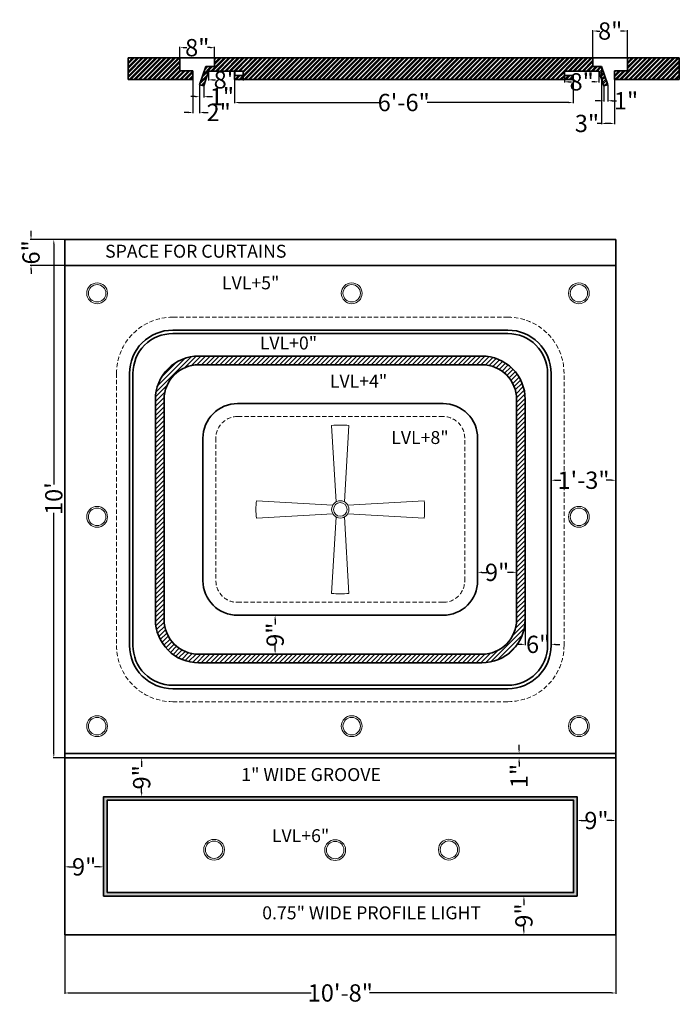
# Model space of a CAD drawing. Units: inches. Extents: x 412 to 565, y 109 to 337.
import ezdxf

# ---------------------------------------------------------------- set-up
doc = ezdxf.new("R2010")
doc.units = ezdxf.units.IN
doc.header["$LTSCALE"] = 2
doc.header["$MEASUREMENT"] = 0
doc.linetypes.add('DASHED', pattern=[0.75, 0.5, -0.25])
for name, color, linetype, lineweight in [('A-ANNO-DIMS', 2, 'Continuous', 18), ('A-ANNO-TEXT', 7, 'Continuous', 18), ('A-CLNG', 7, 'Continuous', 35), ('A-CLNG-LITE', 30, 'DASHED', 18), ('A-CLNG-PATT', 8, 'Continuous', 13), ('A-SECT', 7, 'Continuous', 35), ('E-FANS', 4, 'Continuous', 18), ('E-LITE', 3, 'Continuous', 18)]:
    doc.layers.add(name, color=color, linetype=linetype, lineweight=lineweight)
doc.styles.get("Standard").update_dxf_attribs({"font": 'arial.ttf'})
doc.dimstyles.get("Standard").update_dxf_attribs({"dimtxt": 4, "dimasz": 1, "dimexe": 0.18, "dimexo": 0.0625, "dimgap": 0.09, "dimtad": 0, "dimdec": 0, "dimzin": 0, "dimdsep": 46, "dimlunit": 4, "dimtxsty": 'Standard', "dimcen": 0.09, "dimadec": 0, "dimazin": 0, "dimtfac": 1, "dimtdec": 0, "dimtofl": 0, "dimtmove": 0, "dimatfit": 3, "dimfxl": 1, "dimtolj": 1, "dimtzin": 0, "dimarcsym": 0})

# ---------------------------------------------------------------- blocks, each defined once
blk = doc.blocks.new('*D1')
at = {"layer": 'A-ANNO-DIMS', "color": 0, "lineweight": -2, "transparency": 16777216}
for p, q in [((535.11, 254.83), (535.11, 229.97)), ((550.11, 236.95), (550.11, 229.97)), ((536.11, 230.15), (537.39, 230.15)), ((549.11, 230.15), (547.83, 230.15))]:
    blk.add_line(p, q, dxfattribs=at)
at = {"layer": 'A-ANNO-DIMS', "color": 0, "transparency": 16777216}
for points in [[(536.11, 230.31), (536.11, 229.98), (535.11, 230.15)], [(549.11, 230.31), (549.11, 229.98), (550.11, 230.15)]]:
    blk.add_solid(points, dxfattribs=at)
at = {"layer": 'Defpoints', "color": 0, "transparency": 16777216}
for p in [(535.11, 254.89), (550.11, 237.01), (535.11, 230.15)]:
    blk.add_point(p, dxfattribs=at)
at = {"layer": 'A-ANNO-DIMS', "color": 0, "transparency": 16777216, "insert": (542.61, 230.15), "char_height": 4, "attachment_point": 5}
blk.add_mtext('\\A1;1\'-3"', dxfattribs=at)
blk = doc.blocks.new('*D2')
at = {"layer": 'A-ANNO-DIMS', "color": 0, "lineweight": -2, "transparency": 16777216}
for p, q in [((529.11, 197.83), (529.11, 191.98)), ((528.11, 192.16), (527.11, 192.16)), ((535.11, 191.95), (535.11, 192.34)), ((536.11, 192.16), (537.11, 192.16))]:
    blk.add_line(p, q, dxfattribs=at)
at = {"layer": 'A-ANNO-DIMS', "color": 0, "transparency": 16777216}
for points in [[(528.11, 192.33), (528.11, 192), (529.11, 192.16)], [(536.11, 192.33), (536.11, 192), (535.11, 192.16)]]:
    blk.add_solid(points, dxfattribs=at)
at = {"layer": 'Defpoints', "color": 0, "transparency": 16777216}
for p in [(529.11, 197.89), (529.11, 192.16), (535.11, 191.89)]:
    blk.add_point(p, dxfattribs=at)
at = {"layer": 'A-ANNO-DIMS', "color": 0, "transparency": 16777216, "insert": (532.11, 192.16), "char_height": 4, "attachment_point": 5}
blk.add_mtext('\\A1;6"', dxfattribs=at)
blk = doc.blocks.new('*D3')
at = {"layer": 'A-ANNO-DIMS', "color": 0, "lineweight": -2, "transparency": 16777216}
for p, q in [((518.11, 206.95), (518.11, 209.01)), ((519.11, 208.83), (520.22, 208.83)), ((526.11, 208.83), (525, 208.83)), ((527.11, 197.95), (527.11, 209.01))]:
    blk.add_line(p, q, dxfattribs=at)
at = {"layer": 'A-ANNO-DIMS', "color": 0, "transparency": 16777216}
for points in [[(519.11, 209), (519.11, 208.67), (518.11, 208.83)], [(526.11, 209), (526.11, 208.67), (527.11, 208.83)]]:
    blk.add_solid(points, dxfattribs=at)
at = {"layer": 'Defpoints', "color": 0, "transparency": 16777216}
for p in [(527.11, 208.83), (518.11, 206.89), (527.11, 197.89)]:
    blk.add_point(p, dxfattribs=at)
at = {"layer": 'A-ANNO-DIMS', "color": 0, "transparency": 16777216, "insert": (522.61, 208.83), "char_height": 4, "attachment_point": 5}
blk.add_mtext('\\A1;9"', dxfattribs=at)
blk = doc.blocks.new('*D4')
at = {"layer": 'A-ANNO-DIMS', "color": 0, "lineweight": -2, "transparency": 16777216}
for p, q in [((462.57, 198.89), (471.4, 198.89)), ((471.22, 197.89), (471.22, 196.78)), ((471.22, 190.89), (471.22, 192)), ((453.57, 189.89), (471.4, 189.89))]:
    blk.add_line(p, q, dxfattribs=at)
at = {"layer": 'A-ANNO-DIMS', "color": 0, "transparency": 16777216}
for points in [[(471.05, 197.89), (471.39, 197.89), (471.22, 198.89)], [(471.05, 190.89), (471.39, 190.89), (471.22, 189.89)]]:
    blk.add_solid(points, dxfattribs=at)
at = {"layer": 'Defpoints', "color": 0, "transparency": 16777216}
for p in [(462.51, 198.89), (471.22, 198.89), (453.51, 189.89)]:
    blk.add_point(p, dxfattribs=at)
at = {"layer": 'A-ANNO-DIMS', "color": 0, "transparency": 16777216, "insert": (471.22, 194.39), "char_height": 4, "attachment_point": 5, "rotation": 90}
blk.add_mtext('\\A1;9"', dxfattribs=at)
blk = doc.blocks.new('*D5')
at = {"layer": 'A-ANNO-DIMS', "color": 0, "lineweight": -2, "transparency": 16777216}
for p, q in [((422.57, 165.89), (440.5, 165.89)), ((440.32, 164.89), (440.32, 163.78)), ((440.32, 157.89), (440.32, 159)), ((431.57, 156.89), (440.5, 156.89))]:
    blk.add_line(p, q, dxfattribs=at)
at = {"layer": 'A-ANNO-DIMS', "color": 0, "transparency": 16777216}
for points in [[(440.16, 164.89), (440.49, 164.89), (440.32, 165.89)], [(440.16, 157.89), (440.49, 157.89), (440.32, 156.89)]]:
    blk.add_solid(points, dxfattribs=at)
at = {"layer": 'Defpoints', "color": 0, "transparency": 16777216}
for p in [(422.51, 165.89), (431.51, 156.89), (440.32, 156.89)]:
    blk.add_point(p, dxfattribs=at)
at = {"layer": 'A-ANNO-DIMS', "color": 0, "transparency": 16777216, "insert": (440.32, 161.39), "char_height": 4, "attachment_point": 5, "rotation": 90}
blk.add_mtext('\\A1;9"', dxfattribs=at)
blk = doc.blocks.new('*D6')
at = {"layer": 'A-ANNO-DIMS', "color": 0, "lineweight": -2, "transparency": 16777216}
for p, q in [((550.11, 165.83), (550.11, 151.21)), ((541.11, 156.83), (541.11, 151.21)), ((542.11, 151.39), (543.22, 151.39)), ((549.11, 151.39), (548, 151.39))]:
    blk.add_line(p, q, dxfattribs=at)
at = {"layer": 'A-ANNO-DIMS', "color": 0, "transparency": 16777216}
for points in [[(542.11, 151.56), (542.11, 151.22), (541.11, 151.39)], [(549.11, 151.56), (549.11, 151.22), (550.11, 151.39)]]:
    blk.add_solid(points, dxfattribs=at)
at = {"layer": 'Defpoints', "color": 0, "transparency": 16777216}
for p in [(550.11, 165.89), (541.11, 156.89), (541.11, 151.39)]:
    blk.add_point(p, dxfattribs=at)
at = {"layer": 'A-ANNO-DIMS', "color": 0, "transparency": 16777216, "insert": (545.61, 151.39), "char_height": 4, "attachment_point": 5}
blk.add_mtext('\\A1;9"', dxfattribs=at)
blk = doc.blocks.new('*D7')
at = {"layer": 'A-ANNO-DIMS', "color": 0, "lineweight": -2, "transparency": 16777216}
for p, q in [((541.05, 133.89), (528.64, 133.89)), ((528.82, 132.89), (528.82, 131.78)), ((528.82, 125.89), (528.82, 127)), ((550.05, 124.89), (528.64, 124.89))]:
    blk.add_line(p, q, dxfattribs=at)
at = {"layer": 'A-ANNO-DIMS', "color": 0, "transparency": 16777216}
for points in [[(528.65, 132.89), (528.98, 132.89), (528.82, 133.89)], [(528.65, 125.89), (528.98, 125.89), (528.82, 124.89)]]:
    blk.add_solid(points, dxfattribs=at)
at = {"layer": 'Defpoints', "color": 0, "transparency": 16777216}
for p in [(528.82, 133.89), (541.11, 133.89), (550.11, 124.89)]:
    blk.add_point(p, dxfattribs=at)
at = {"layer": 'A-ANNO-DIMS', "color": 0, "transparency": 16777216, "insert": (528.82, 129.39), "char_height": 4, "attachment_point": 5, "rotation": 90}
blk.add_mtext('\\A1;9"', dxfattribs=at)
blk = doc.blocks.new('*D8')
at = {"layer": 'A-ANNO-DIMS', "color": 0, "lineweight": -2, "transparency": 16777216}
for p, q in [((422.51, 124.95), (422.51, 140.84)), ((423.51, 140.66), (424.62, 140.66)), ((430.51, 140.66), (429.4, 140.66)), ((431.51, 133.95), (431.51, 140.84))]:
    blk.add_line(p, q, dxfattribs=at)
at = {"layer": 'A-ANNO-DIMS', "color": 0, "transparency": 16777216}
for points in [[(423.51, 140.83), (423.51, 140.49), (422.51, 140.66)], [(430.51, 140.83), (430.51, 140.49), (431.51, 140.66)]]:
    blk.add_solid(points, dxfattribs=at)
at = {"layer": 'Defpoints', "color": 0, "transparency": 16777216}
for p in [(422.51, 140.66), (431.51, 133.89), (422.51, 124.89)]:
    blk.add_point(p, dxfattribs=at)
at = {"layer": 'A-ANNO-DIMS', "color": 0, "transparency": 16777216, "insert": (427.01, 140.66), "char_height": 4, "attachment_point": 5}
blk.add_mtext('\\A1;9"', dxfattribs=at)
blk = doc.blocks.new('*D9')
at = {"layer": 'A-ANNO-DIMS', "color": 0, "lineweight": -2, "transparency": 16777216}
for p, q in [((527.7, 167.89), (527.7, 168.89)), ((550.05, 166.89), (527.52, 166.89)), ((550.05, 165.89), (527.52, 165.89)), ((527.7, 164.89), (527.7, 163.89))]:
    blk.add_line(p, q, dxfattribs=at)
at = {"layer": 'A-ANNO-DIMS', "color": 0, "transparency": 16777216}
for points in [[(527.53, 167.89), (527.87, 167.89), (527.7, 166.89)], [(527.53, 164.89), (527.87, 164.89), (527.7, 165.89)]]:
    blk.add_solid(points, dxfattribs=at)
at = {"layer": 'Defpoints', "color": 0, "transparency": 16777216}
for p in [(550.11, 166.89), (527.7, 165.89), (550.11, 165.89)]:
    blk.add_point(p, dxfattribs=at)
at = {"layer": 'A-ANNO-DIMS', "color": 0, "transparency": 16777216, "insert": (527.7, 161.69), "char_height": 4, "attachment_point": 5, "rotation": 90}
blk.add_mtext('\\A1;1"', dxfattribs=at)
blk = doc.blocks.new('*D10')
at = {"layer": 'A-ANNO-DIMS', "color": 0, "lineweight": -2, "transparency": 16777216}
for p, q in [((414.71, 286.89), (414.71, 287.89)), ((422.45, 285.89), (414.53, 285.89)), ((422.45, 279.89), (414.53, 279.89)), ((414.71, 278.89), (414.71, 277.89))]:
    blk.add_line(p, q, dxfattribs=at)
at = {"layer": 'A-ANNO-DIMS', "color": 0, "transparency": 16777216}
for points in [[(414.54, 286.89), (414.88, 286.89), (414.71, 285.89)], [(414.54, 278.89), (414.88, 278.89), (414.71, 279.89)]]:
    blk.add_solid(points, dxfattribs=at)
at = {"layer": 'Defpoints', "color": 0, "transparency": 16777216}
for p in [(422.51, 285.89), (414.71, 279.89), (422.51, 279.89)]:
    blk.add_point(p, dxfattribs=at)
at = {"layer": 'A-ANNO-DIMS', "color": 0, "transparency": 16777216, "insert": (414.71, 282.89), "char_height": 4, "attachment_point": 5, "rotation": 90}
blk.add_mtext('\\A1;6"', dxfattribs=at)
blk = doc.blocks.new('*D11')
at = {"layer": 'A-ANNO-DIMS', "color": 0, "lineweight": -2, "transparency": 16777216}
for p, q in [((422.45, 285.89), (419.8, 285.89)), ((419.98, 284.89), (419.98, 229.18)), ((419.98, 166.89), (419.98, 222.59)), ((422.45, 165.89), (419.8, 165.89))]:
    blk.add_line(p, q, dxfattribs=at)
at = {"layer": 'A-ANNO-DIMS', "color": 0, "transparency": 16777216}
for points in [[(419.82, 284.89), (420.15, 284.89), (419.98, 285.89)], [(419.82, 166.89), (420.15, 166.89), (419.98, 165.89)]]:
    blk.add_solid(points, dxfattribs=at)
at = {"layer": 'Defpoints', "color": 0, "transparency": 16777216}
for p in [(422.51, 285.89), (419.98, 165.89), (422.51, 165.89)]:
    blk.add_point(p, dxfattribs=at)
at = {"layer": 'A-ANNO-DIMS', "color": 0, "transparency": 16777216, "insert": (419.98, 225.89), "char_height": 4, "attachment_point": 5, "rotation": 90}
blk.add_mtext("\\A1;10'", dxfattribs=at)
blk = doc.blocks.new('*D12')
at = {"layer": 'A-ANNO-DIMS', "color": 0, "lineweight": -2, "transparency": 16777216}
for p, q in [((422.51, 124.83), (422.51, 111.29)), ((550.11, 124.83), (550.11, 111.29)), ((423.51, 111.47), (479.54, 111.47)), ((549.11, 111.47), (493.08, 111.47))]:
    blk.add_line(p, q, dxfattribs=at)
at = {"layer": 'A-ANNO-DIMS', "color": 0, "transparency": 16777216}
for points in [[(423.51, 111.63), (423.51, 111.3), (422.51, 111.47)], [(549.11, 111.63), (549.11, 111.3), (550.11, 111.47)]]:
    blk.add_solid(points, dxfattribs=at)
at = {"layer": 'Defpoints', "color": 0, "transparency": 16777216}
for p in [(422.51, 124.89), (550.11, 124.89), (550.11, 111.47)]:
    blk.add_point(p, dxfattribs=at)
at = {"layer": 'A-ANNO-DIMS', "color": 0, "transparency": 16777216, "insert": (486.31, 111.47), "char_height": 4, "attachment_point": 5}
blk.add_mtext('\\A1;10\'-8"', dxfattribs=at)
blk = doc.blocks.new('*D13')
at = {"layer": 'A-ANNO-DIMS', "color": 0, "lineweight": -2, "transparency": 16777216}
for p, q in [((461.8, 322.85), (461.8, 317.4)), ((540.19, 322.85), (540.19, 317.4)), ((462.8, 317.58), (495.58, 317.58)), ((539.19, 317.58), (506.41, 317.58))]:
    blk.add_line(p, q, dxfattribs=at)
at = {"layer": 'A-ANNO-DIMS', "color": 0, "transparency": 16777216}
for points in [[(462.8, 317.74), (462.8, 317.41), (461.8, 317.58)], [(539.19, 317.74), (539.19, 317.41), (540.19, 317.58)]]:
    blk.add_solid(points, dxfattribs=at)
at = {"layer": 'Defpoints', "color": 0, "transparency": 16777216}
for p in [(461.8, 322.91), (540.19, 322.91), (461.8, 317.58)]:
    blk.add_point(p, dxfattribs=at)
at = {"layer": 'A-ANNO-DIMS', "color": 0, "transparency": 16777216, "insert": (500.99, 317.58), "char_height": 4, "attachment_point": 5}
blk.add_mtext('\\A1;6\'-6"', dxfattribs=at)
blk = doc.blocks.new('*D14')
at = {"layer": 'A-ANNO-DIMS', "color": 0, "lineweight": -2, "transparency": 16777216}
for p, q in [((453.73, 321.63), (453.73, 318.76)), ((454.7, 321.37), (454.7, 318.76)), ((452.73, 318.94), (451.73, 318.94)), ((455.7, 318.94), (456.7, 318.94))]:
    blk.add_line(p, q, dxfattribs=at)
at = {"layer": 'A-ANNO-DIMS', "color": 0, "transparency": 16777216}
for points in [[(452.73, 319.1), (452.73, 318.77), (453.73, 318.94)], [(455.7, 319.1), (455.7, 318.77), (454.7, 318.94)]]:
    blk.add_solid(points, dxfattribs=at)
at = {"layer": 'Defpoints', "color": 0, "transparency": 16777216}
for p in [(453.73, 321.7), (454.7, 321.44), (454.7, 318.94)]:
    blk.add_point(p, dxfattribs=at)
at = {"layer": 'A-ANNO-DIMS', "color": 0, "transparency": 16777216, "insert": (458.9, 318.94), "char_height": 4, "attachment_point": 5}
blk.add_mtext('\\A1;1"', dxfattribs=at)
blk = doc.blocks.new('*D15')
at = {"layer": 'A-ANNO-DIMS', "color": 0, "lineweight": -2, "transparency": 16777216}
for p, q in [((455.8, 324.78), (455.8, 322.65)), ((463.8, 324.78), (463.8, 322.65)), ((456.8, 322.83), (457.41, 322.83)), ((462.8, 322.83), (462.19, 322.83))]:
    blk.add_line(p, q, dxfattribs=at)
at = {"layer": 'A-ANNO-DIMS', "color": 0, "transparency": 16777216}
for points in [[(456.8, 322.99), (456.8, 322.66), (455.8, 322.83)], [(462.8, 322.99), (462.8, 322.66), (463.8, 322.83)]]:
    blk.add_solid(points, dxfattribs=at)
at = {"layer": 'Defpoints', "color": 0, "transparency": 16777216}
for p in [(455.8, 324.84), (463.8, 324.84), (463.8, 322.83)]:
    blk.add_point(p, dxfattribs=at)
at = {"layer": 'A-ANNO-DIMS', "color": 0, "transparency": 16777216, "insert": (459.8, 322.83), "char_height": 4, "attachment_point": 5}
blk.add_mtext('\\A1;8"', dxfattribs=at)
blk = doc.blocks.new('*D16')
at = {"layer": 'A-ANNO-DIMS', "color": 0, "lineweight": -2, "transparency": 16777216}
for p, q in [((452.19, 322.85), (452.19, 315.09)), ((453.73, 321.63), (453.73, 315.09)), ((451.19, 315.27), (450.19, 315.27)), ((454.73, 315.27), (455.73, 315.27))]:
    blk.add_line(p, q, dxfattribs=at)
at = {"layer": 'A-ANNO-DIMS', "color": 0, "transparency": 16777216}
for points in [[(451.19, 315.44), (451.19, 315.1), (452.19, 315.27)], [(454.73, 315.44), (454.73, 315.1), (453.73, 315.27)]]:
    blk.add_solid(points, dxfattribs=at)
at = {"layer": 'Defpoints', "color": 0, "transparency": 16777216}
for p in [(452.19, 322.91), (453.73, 321.7), (453.73, 315.27)]:
    blk.add_point(p, dxfattribs=at)
at = {"layer": 'A-ANNO-DIMS', "color": 0, "transparency": 16777216, "insert": (458.15, 315.27), "char_height": 4, "attachment_point": 5}
blk.add_mtext('\\A1;2"', dxfattribs=at)
blk = doc.blocks.new('*D17')
at = {"layer": 'A-ANNO-DIMS', "color": 0, "lineweight": -2, "transparency": 16777216}
for p, q in [((449.19, 327.97), (449.19, 330.46)), ((450.19, 330.28), (450.8, 330.28)), ((456.19, 330.28), (455.59, 330.28)), ((457.19, 327.97), (457.19, 330.46))]:
    blk.add_line(p, q, dxfattribs=at)
at = {"layer": 'A-ANNO-DIMS', "color": 0, "transparency": 16777216}
for points in [[(450.19, 330.45), (450.19, 330.11), (449.19, 330.28)], [(456.19, 330.45), (456.19, 330.11), (457.19, 330.28)]]:
    blk.add_solid(points, dxfattribs=at)
at = {"layer": 'Defpoints', "color": 0, "transparency": 16777216}
for p in [(457.19, 330.28), (449.19, 327.91), (457.19, 327.91)]:
    blk.add_point(p, dxfattribs=at)
at = {"layer": 'A-ANNO-DIMS', "color": 0, "transparency": 16777216, "insert": (453.19, 330.28), "char_height": 4, "attachment_point": 5}
blk.add_mtext('\\A1;8"', dxfattribs=at)
blk = doc.blocks.new('*D18')
at = {"layer": 'A-ANNO-DIMS', "color": 0, "lineweight": -2, "transparency": 16777216}
for p, q in [((544.79, 327.97), (544.79, 334.31)), ((545.79, 334.13), (546.4, 334.13)), ((551.79, 334.13), (551.19, 334.13)), ((552.79, 327.97), (552.79, 334.31))]:
    blk.add_line(p, q, dxfattribs=at)
at = {"layer": 'A-ANNO-DIMS', "color": 0, "transparency": 16777216}
for points in [[(545.79, 334.29), (545.79, 333.96), (544.79, 334.13)], [(551.79, 334.29), (551.79, 333.96), (552.79, 334.13)]]:
    blk.add_solid(points, dxfattribs=at)
at = {"layer": 'Defpoints', "color": 0, "transparency": 16777216}
for p in [(552.79, 334.13), (544.79, 327.91), (552.79, 327.91)]:
    blk.add_point(p, dxfattribs=at)
at = {"layer": 'A-ANNO-DIMS', "color": 0, "transparency": 16777216, "insert": (548.79, 334.13), "char_height": 4, "attachment_point": 5}
blk.add_mtext('\\A1;8"', dxfattribs=at)
blk = doc.blocks.new('*D19')
at = {"layer": 'A-ANNO-DIMS', "color": 0, "lineweight": -2, "transparency": 16777216}
for p, q in [((546.79, 325.85), (546.79, 312.56)), ((549.79, 324.85), (549.79, 312.56)), ((546.79, 312.74), (545.79, 312.74)), ((548.79, 312.74), (547.79, 312.74))]:
    blk.add_line(p, q, dxfattribs=at)
at = {"layer": 'A-ANNO-DIMS', "color": 0, "transparency": 16777216}
for points in [[(547.79, 312.91), (547.79, 312.57), (546.79, 312.74)], [(548.79, 312.91), (548.79, 312.57), (549.79, 312.74)]]:
    blk.add_solid(points, dxfattribs=at)
at = {"layer": 'Defpoints', "color": 0, "transparency": 16777216}
for p in [(546.79, 325.91), (549.79, 324.91), (546.79, 312.74)]:
    blk.add_point(p, dxfattribs=at)
at = {"layer": 'A-ANNO-DIMS', "color": 0, "transparency": 16777216, "insert": (543.41, 312.74), "char_height": 4, "attachment_point": 5}
blk.add_mtext('\\A1;3"', dxfattribs=at)
blk = doc.blocks.new('*D20')
at = {"layer": 'A-ANNO-DIMS', "color": 0, "lineweight": -2, "transparency": 16777216}
for p, q in [((547.29, 321.37), (547.29, 317.81)), ((548.26, 321.63), (548.26, 317.81)), ((546.29, 317.99), (545.29, 317.99)), ((549.26, 317.99), (550.26, 317.99))]:
    blk.add_line(p, q, dxfattribs=at)
at = {"layer": 'A-ANNO-DIMS', "color": 0, "transparency": 16777216}
for points in [[(546.29, 318.16), (546.29, 317.83), (547.29, 317.99)], [(549.26, 318.16), (549.26, 317.83), (548.26, 317.99)]]:
    blk.add_solid(points, dxfattribs=at)
at = {"layer": 'Defpoints', "color": 0, "transparency": 16777216}
for p in [(547.29, 321.44), (548.26, 321.7), (548.26, 317.99)]:
    blk.add_point(p, dxfattribs=at)
at = {"layer": 'A-ANNO-DIMS', "color": 0, "transparency": 16777216, "insert": (552.46, 317.99), "char_height": 4, "attachment_point": 5}
blk.add_mtext('\\A1;1"', dxfattribs=at)
blk = doc.blocks.new('*D21')
at = {"layer": 'A-ANNO-DIMS', "color": 0, "lineweight": -2, "transparency": 16777216}
for p, q in [((538.19, 324.78), (538.19, 322.19)), ((546.19, 324.78), (546.19, 322.19)), ((539.19, 322.37), (539.8, 322.37)), ((545.19, 322.37), (544.58, 322.37))]:
    blk.add_line(p, q, dxfattribs=at)
at = {"layer": 'A-ANNO-DIMS', "color": 0, "transparency": 16777216}
for points in [[(539.19, 322.54), (539.19, 322.2), (538.19, 322.37)], [(545.19, 322.54), (545.19, 322.2), (546.19, 322.37)]]:
    blk.add_solid(points, dxfattribs=at)
at = {"layer": 'Defpoints', "color": 0, "transparency": 16777216}
for p in [(538.19, 324.84), (546.19, 324.84), (538.19, 322.37)]:
    blk.add_point(p, dxfattribs=at)
at = {"layer": 'A-ANNO-DIMS', "color": 0, "transparency": 16777216, "insert": (542.19, 322.37), "char_height": 4, "attachment_point": 5}
blk.add_mtext('\\A1;8"', dxfattribs=at)
blk = doc.blocks.new('LIGHT-DOWN')
for radius in [2.41, 2.02]:
    blk.add_circle((2.41, 2.41), radius)
blk = doc.blocks.new('FAN-BLADE')
for p, q in [((0, 2.98), (17.69, 4)), ((0, 1.01), (17.69, 0))]:
    blk.add_line(p, q)
blk.add_arc((-1.74, 2), 19.53, 354.1232, 5.8768)

msp = doc.modelspace()

# ---------------------------------------------------------------- hatches: boundary and pattern name
at = {"layer": 'A-CLNG-PATT'}
h = msp.add_hatch(dxfattribs=at)
h.set_pattern_fill('ANSI32', color=256, scale=2)
h.paths.add_polyline_path([(449.19, 327.91), (437.19, 327.91), (437.19, 322.91), (452.19, 322.91), (452.19, 323.91), (452.19, 324.91), (449.19, 324.91)])
h.paths.add_polyline_path([(546.79, 325.91), (544.79, 325.91), (544.79, 327.91), (457.19, 327.91), (457.19, 325.91), (455.19, 325.91), (453.73, 321.7), (454.7, 321.44), (455.8, 324.84), (463.8, 324.84), (463.8, 323.84), (461.8, 323.84), (461.8, 322.91), (540.19, 322.91), (540.19, 323.84), (538.19, 323.84), (538.19, 324.84), (546.19, 324.84), (547.29, 321.44), (548.26, 321.7)])
h.paths.add_polyline_path([(564.79, 327.91), (552.79, 327.91), (552.79, 324.91), (549.79, 324.91), (549.79, 323.91), (549.79, 322.91), (564.79, 322.91)])
h = msp.add_hatch(dxfattribs=at)
h.set_pattern_fill('ANSI31', color=256, scale=6)
h.paths.add_polyline_path([(519.11, 258.89), (453.51, 258.89, 0.414214), (443.51, 248.89), (443.51, 197.89, 0.414214), (453.51, 187.89), (519.11, 187.89, 0.414214), (529.11, 197.89), (529.11, 248.89, 0.414214)])
h.paths.add_polyline_path([(453.51, 256.89), (519.11, 256.89, -0.414214), (527.11, 248.89), (527.11, 197.89, -0.414214), (519.11, 189.89), (453.51, 189.89, -0.414214), (445.51, 197.89), (445.51, 248.89, -0.414214)], flags=16)
h.paths.add_polyline_path([(462.51, 247.89), (510.11, 247.89, -0.414214), (518.11, 239.89), (518.11, 206.89, -0.414214), (510.11, 198.89), (462.51, 198.89, -0.414214), (454.51, 206.89), (454.51, 239.89, -0.414214)], flags=0)
h = msp.add_hatch(color=256, dxfattribs=at)
h.dxf.hatch_style = 1
h.paths.add_polyline_path([(541.11, 156.89), (431.51, 156.89), (431.51, 133.89), (541.11, 133.89)])
h.paths.add_polyline_path([(540.31, 156.09), (540.31, 134.69), (432.31, 134.69), (432.31, 156.09)], flags=16)

# ---------------------------------------------------------------- linework, layer by layer
at = {"layer": 'A-CLNG'}
for p, q in [((422.51, 285.89), (422.51, 124.89)), ((550.11, 285.89), (422.51, 285.89)), ((550.11, 124.89), (550.11, 285.89)), ((550.11, 279.89), (422.51, 279.89)), ((422.51, 166.89), (550.11, 166.89)), ((422.51, 165.89), (550.11, 165.89)), ((422.51, 124.89), (550.11, 124.89))]:
    msp.add_line(p, q, dxfattribs=at)
for points in [[(437.51, 191.89, 0.414214), (447.51, 181.89), (525.11, 181.89, 0.414214), (535.11, 191.89), (535.11, 254.89, 0.414214), (525.11, 264.89), (447.51, 264.89, 0.414214), (437.51, 254.89)], [(438.31, 191.89, 0.414214), (447.51, 182.69), (525.11, 182.69, 0.414214), (534.31, 191.89), (534.31, 254.89, 0.414214), (525.11, 264.09), (447.51, 264.09, 0.414214), (438.31, 254.89)], [(529.11, 248.89, 0.414214), (519.11, 258.89), (453.51, 258.89, 0.414214), (443.51, 248.89), (443.51, 197.89, 0.414214), (453.51, 187.89), (519.11, 187.89, 0.414214), (529.11, 197.89)], [(527.11, 248.89, 0.414214), (519.11, 256.89), (453.51, 256.89, 0.414214), (445.51, 248.89), (445.51, 197.89, 0.414214), (453.51, 189.89), (519.11, 189.89, 0.414214), (527.11, 197.89)], [(510.11, 198.89, 0.414214), (518.11, 206.89), (518.11, 239.89, 0.414214), (510.11, 247.89), (462.51, 247.89, 0.414214), (454.51, 239.89), (454.51, 206.89, 0.414214), (462.51, 198.89)]]:
    msp.add_lwpolyline(points, format="xyb", close=True, dxfattribs=at)
for points in [[(431.51, 133.89), (541.11, 133.89), (541.11, 156.89), (431.51, 156.89)], [(432.31, 134.69), (540.31, 134.69), (540.31, 156.09), (432.31, 156.09)]]:
    msp.add_lwpolyline(points, close=True, dxfattribs=at)
at = {"layer": 'A-CLNG-LITE'}
for points in [[(434.51, 191.89, 0.414214), (447.51, 178.89), (525.11, 178.89, 0.414214), (538.11, 191.89), (538.11, 254.89, 0.414214), (525.11, 267.89), (447.51, 267.89, 0.414214), (434.51, 254.89)], [(510.11, 201.89, 0.414214), (515.11, 206.89), (515.11, 239.89, 0.414214), (510.11, 244.89), (462.51, 244.89, 0.414214), (457.51, 239.89), (457.51, 206.89, 0.414214), (462.51, 201.89)]]:
    msp.add_lwpolyline(points, format="xyb", close=True, dxfattribs=at)
at = {"layer": 'A-SECT'}
for p, q in [((437.19, 327.91), (564.79, 327.91)), ((437.19, 322.91), (437.19, 327.91)), ((449.19, 324.91), (449.19, 327.91)), ((455.19, 325.91), (453.73, 321.7)), ((457.19, 325.91), (455.19, 325.91)), ((457.19, 327.91), (457.19, 325.91)), ((544.79, 327.91), (544.79, 325.91)), ((544.79, 325.91), (546.79, 325.91)), ((546.79, 325.91), (548.26, 321.7)), ((552.79, 324.91), (552.79, 327.91)), ((564.79, 327.91), (564.79, 322.91)), ((564.79, 322.91), (564.79, 327.91)), ((452.19, 324.91), (449.19, 324.91)), ((452.19, 323.91), (452.19, 324.91)), ((452.19, 322.91), (452.19, 323.91)), ((454.7, 321.44), (455.8, 324.84)), ((455.8, 324.84), (463.8, 324.84)), ((463.8, 323.84), (461.8, 323.84)), ((461.8, 323.84), (461.8, 322.91)), ((463.8, 324.84), (463.8, 323.84)), ((546.19, 324.84), (538.19, 324.84)), ((538.19, 324.84), (538.19, 323.84)), ((538.19, 323.84), (540.19, 323.84)), ((540.19, 323.84), (540.19, 322.91)), ((547.29, 321.44), (546.19, 324.84)), ((549.79, 323.91), (549.79, 324.91)), ((549.79, 324.91), (552.79, 324.91)), ((549.79, 322.91), (549.79, 323.91)), ((452.19, 322.91), (437.19, 322.91)), ((453.73, 321.7), (454.7, 321.44)), ((540.19, 322.91), (461.8, 322.91)), ((548.26, 321.7), (547.29, 321.44)), ((564.79, 322.91), (549.79, 322.91))]:
    msp.add_line(p, q, dxfattribs=at)
at = {"layer": 'E-FANS'}
for radius in [2, 1.57]:
    msp.add_circle((486.31, 223.39), radius, dxfattribs=at)

# ---------------------------------------------------------------- block references
for p, rotation in [((488.31, 225.13), 90.00000000000011), ((484.57, 225.39), 180), ((484.31, 221.65), 270.0000000000001)]:
    msp.add_blockref('FAN-BLADE', p, dxfattribs=dict(at, rotation=rotation))
msp.add_blockref('FAN-BLADE', (488.05, 221.39), dxfattribs=at)
at = {"layer": 'E-LITE'}
for p in [(427.6, 271.02), (486.54, 271.02), (539.14, 271.02), (427.6, 219.27), (539.14, 219.27), (427.6, 170.82), (486.54, 170.82), (539.14, 170.82), (454.68, 142.21), (482.71, 142.13), (509.04, 142.24)]:
    msp.add_blockref('LIGHT-DOWN', p, dxfattribs=at)

# ---------------------------------------------------------------- texts
at = {"layer": 'A-ANNO-TEXT', "char_height": 3, "attachment_point": 1}
for s, width, insert in [('\\pxqc;SPACE FOR CURTAINS', 60.6714, (422.51, 284.66)), ('\\pxqc;LVL+5"', 23.8117, (453.66, 277.34)), ('\\pxqc;LVL+0"', 23.8117, (462.4, 263.42)), ('\\pxqc;LVL+4"', 23.8117, (478.63, 254.6)), ('\\pxqc;LVL+8"', 23.8117, (492.85, 241.54)), ('\\pxqc;1" WIDE GROOVE', 37.107, (460.99, 163.52)), ('\\pxqc;LVL+6"', 23.8117, (465.21, 149.38)), ('\\pxqc;0.75" WIDE PROFILE LIGHT', 61.9002, (462.61, 131.52))]:
    msp.add_mtext_dynamic_manual_height_columns(s, width=width, gutter_width=15, heights=[0], dxfattribs=dict(at, insert=insert))

# ---------------------------------------------------------------- dimensions: what is measured, and where the dimension line sits
at = {"layer": 'A-ANNO-DIMS'}
for base, p1, p2, picture, middle in [((552.79, 334.13), (544.79, 327.91), (552.79, 327.91), '*D18', (548.79, 334.13)), ((457.19, 330.28), (449.19, 327.91), (457.19, 327.91), '*D17', (453.19, 330.28)), ((546.79, 312.74), (549.79, 324.91), (546.79, 325.91), '*D19', (543.41, 312.74)), ((463.8, 322.83), (455.8, 324.84), (463.8, 324.84), '*D15', (459.8, 322.83)), ((538.19, 322.37), (546.19, 324.84), (538.19, 324.84), '*D21', (542.19, 322.37)), ((453.73, 315.27), (452.19, 322.91), (453.73, 321.7), '*D16', (458.15, 315.27)), ((454.7, 318.94), (453.73, 321.7), (454.7, 321.44), '*D14', (458.9, 318.94)), ((461.8, 317.58), (540.19, 322.91), (461.8, 322.91), '*D13', (500.99, 317.58)), ((548.26, 317.99), (547.29, 321.44), (548.26, 321.7), '*D20', (552.46, 317.99)), ((535.11, 230.15), (550.11, 237.01), (535.11, 254.89), '*D1', (542.61, 230.15)), ((527.11, 208.83), (518.11, 206.89), (527.11, 197.89), '*D3', (522.61, 208.83)), ((529.11, 192.16), (535.11, 191.89), (529.11, 197.89), '*D2', (532.11, 192.16)), ((541.11, 151.39), (550.11, 165.89), (541.11, 156.89), '*D6', (545.61, 151.39)), ((422.51, 140.66), (431.51, 133.89), (422.51, 124.89), '*D8', (427.01, 140.66)), ((550.11, 111.47), (422.51, 124.89), (550.11, 124.89), '*D12', (486.31, 111.47))]:
    dim = msp.add_linear_dim(base=base, p1=p1, p2=p2, dimstyle='Standard', override={"dimclrd": 0, "dimclre": 0, "dimclrt": 0}, dxfattribs=at)
    dim.commit()
    dim.dimension.update_dxf_attribs({"geometry": picture, "text_midpoint": middle})
for base, p1, p2, picture, middle in [((414.71, 279.89), (422.51, 285.89), (422.51, 279.89), '*D10', (414.71, 282.89)), ((419.98, 165.89), (422.51, 285.89), (422.51, 165.89), '*D11', (419.98, 225.89)), ((471.22, 198.89), (453.51, 189.89), (462.51, 198.89), '*D4', (471.22, 194.39)), ((527.7, 165.89), (550.11, 166.89), (550.11, 165.89), '*D9', (527.7, 161.69)), ((440.32, 156.89), (422.51, 165.89), (431.51, 156.89), '*D5', (440.32, 161.39)), ((528.82, 133.89), (550.11, 124.89), (541.11, 133.89), '*D7', (528.82, 129.39))]:
    dim = msp.add_linear_dim(base=base, p1=p1, p2=p2, angle=90, dimstyle='Standard', override={"dimclrd": 0, "dimclre": 0, "dimclrt": 0}, dxfattribs=at)
    dim.commit()
    dim.dimension.update_dxf_attribs({"geometry": picture, "text_midpoint": middle})

doc.saveas('drawing.dxf')
